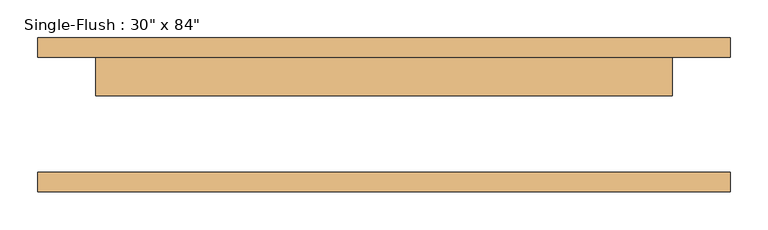
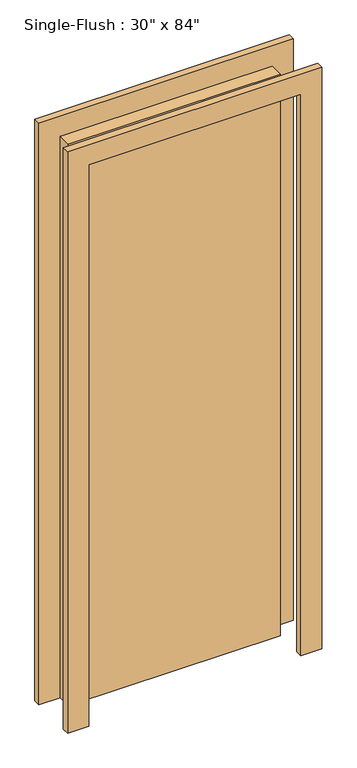
"""IFC4 building model written with IfcOpenShell, lengths in millimetres: door geometry."""

from ifc_helpers import new_model, si_unit, frame, origin, origin_with_axes, place, context, project, spatial, polyline, outline, extrude, source, transform, mapped, element, save


def door_a9addea7(model_context):
    return source(origin(), model_context, "Body", "SweptSolid", [
        extrude(outline(polyline([(2209.8, -457.2), (0.0, -457.2), (0.0, -381.0), (2133.6, -381.0), (2133.6, 381.0), (0.0, 381.0), (0.0, 457.2), (2209.8, 457.2), (2209.8, -457.2)])), frame((0.0, 76.2, 0.0), z_axis=(0.0, 1.0, 0.0), x_axis=(0.0, 0.0, 1.0)), (0.0, 0.0, 1.0), 25.4),
        extrude(outline(polyline([(2209.8, 457.2), (2209.8, -457.2), (0.0, -457.2), (0.0, -381.0), (2133.6, -381.0), (2133.6, 381.0), (0.0, 381.0), (0.0, 457.2), (2209.8, 457.2)])), frame((0.0, -101.6, 0.0), z_axis=(0.0, 1.0, 0.0), x_axis=(0.0, 0.0, 1.0)), (0.0, 0.0, 1.0), 25.4),
        extrude(outline(polyline([(381.0, 25.4), (-381.0, 25.4), (-381.0, 76.2), (381.0, 76.2), (381.0, 25.4)])), origin_with_axes(), (0.0, 0.0, 1.0), 2133.6),
    ])


if __name__ == "__main__":
    model = new_model("IFC4")
    model_context = context("Model", 3, world=origin())
    ifc_project = project(units=[si_unit("LENGTHUNIT", "METRE", prefix="MILLI")], contexts=[model_context])
    site = spatial("IfcSite", under=ifc_project)
    building = spatial("IfcBuilding", under=site)
    placement = place(None, origin())
    door_shape = door_a9addea7(model_context)
    element("IfcDoor", 1, ObjectType="Single-Flush : 30\" x 84\"", at=placement, inside=building, context=model_context, shape_type="MappedRepresentation", body=[
        mapped(door_shape, transform((0.0, 0.0, 0.0), x_axis=(1.0, 0.0, 0.0), y_axis=(0.0, 1.0, 0.0), z_axis=(0.0, 0.0, 1.0))),
    ])
    save(model, "model.ifc")

# Revit data of these elements
# Type "Single-Flush : 30\" x 84\""
#   Type Mark = "4"
#   Construction Type Id = "MDOOR"
#   Assembly Code = "C1020"
#   Analytic Construction = "Metal"
#   Thickness = 0' - 2"
#   Heat Transfer Coefficient (U) = 0.651978 BTU/(h·ft²·°F)
#   Height = 7' - 0"
#   Trim Projection Ext = 0' - 1"
#   Trim Projection Int = 0' - 1"
#   Trim Width = 0' - 3"
#   Width = 2' - 6"
#   Define Thermal Properties by = 1
#   Define Thermal Properties by = 1
#   Door Material = Door - Panel
#   Frame Material = Door - Frame
#   Visual Light Transmittance = 0
#   Solar Heat Gain Coefficient = 0
#   Function = (empty or 0)
#   Wall Closure = (empty or 0)
# Element 1 (IfcDoor, "Single-Flush : 30\" x 84\"")
#   Materials on its faces: "Door - Frame", "Door - Panel"
# Materials
#   "Door - Panel": class "Wood", colour RGB 210 159 95, transparency 0, Cost = 0
#   "Door - Frame": colour RGB 118 70 51, transparency 0, Cost = 0
